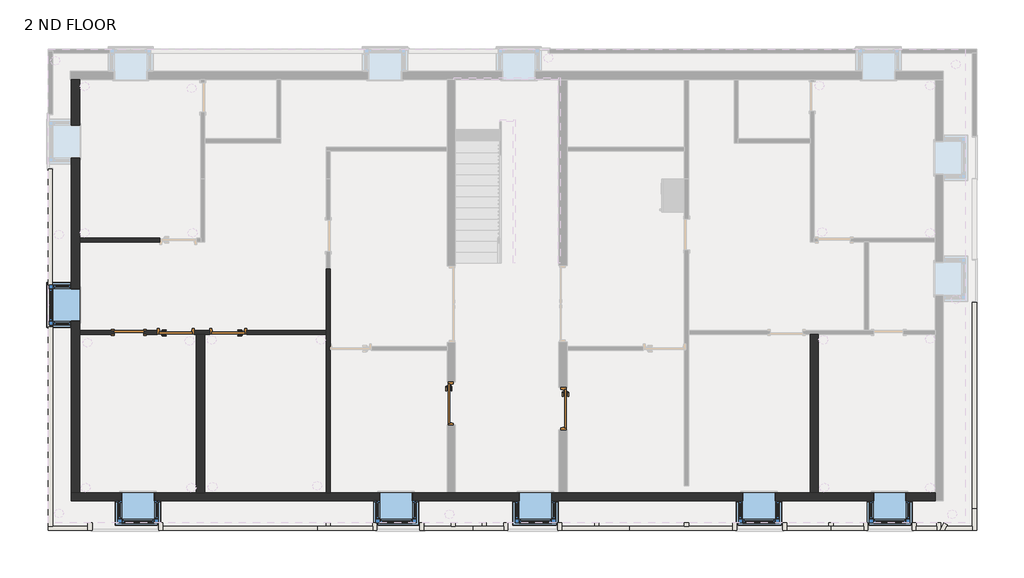
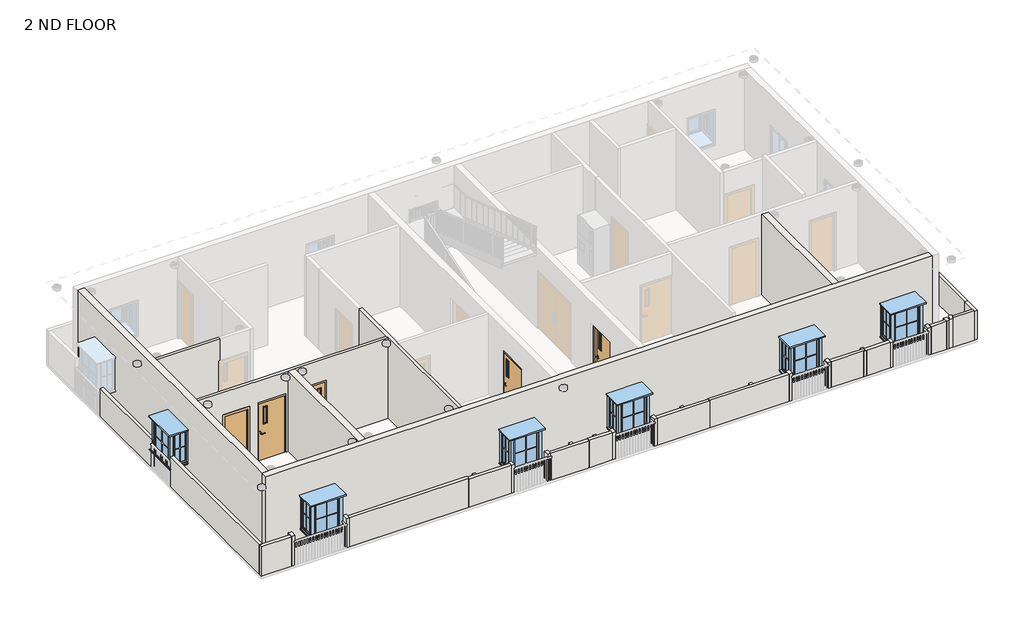
# One storey, part 1 of 7: 40 walls, 6 windows, 5 doors.
"""IFC4 building model written with IfcOpenShell, lengths in millimetres."""

from ifc_helpers import new_model, si_unit, frame, origin, place, context, project, spatial, polyline, outline, extrude, faceted_brep, transform, mapped, element, save
from components import door_586e558e, door_7d8f8091, door_passage_single_vision_lite_3_x7_440dd290, door_passage_single_vision_lite_3_x7_38248cdf, door_d141acb4, window_bay_casement_box_90_degree_angle_center_fixed_4_x3_2dea7aab

model = new_model("IFC4")

# Units and contexts
model_context = context("Model", 3, world=origin())
ifc_project = project(units=[si_unit("LENGTHUNIT", "METRE", prefix="MILLI")], contexts=[model_context])

# Site, building, storey
site = spatial("IfcSite", under=ifc_project)
building = spatial("IfcBuilding", under=site)
storey = spatial("IfcBuildingStorey", under=building, Name="2 ND FLOOR", Elevation=6400.8)

# Doors
placement = place(None, origin())
door_shape = door_586e558e(model_context)
element("IfcDoor", 1, ObjectType="Door-Passage-Single-Vision_Lite : 3'6\"X7' 2", at=placement, inside=storey, context=model_context, shape_type="MappedRepresentation", body=[
    mapped(door_shape, transform((1116.1432011, -1461.3932193, 6400.8), x_axis=(0.0, -1.0, 0.0), y_axis=(1.0, 0.0, 0.0), z_axis=(0.0, 0.0, 1.0))),
])
door_2_shape = door_7d8f8091(model_context)
element("IfcDoor", 2, ObjectType="Door-Passage-Single-Vision_Lite : 3'7\"X7' 3", at=placement, inside=storey, context=model_context, shape_type="MappedRepresentation", body=[
    mapped(door_2_shape, transform((-1956.7487998, -1318.7421379, 6400.8), x_axis=(0.0, -1.0, 0.0), y_axis=(1.0, 0.0, 0.0), z_axis=(0.0, 0.0, 1.0))),
])
door_passage_single_vision_lite_3_x7_shape = door_passage_single_vision_lite_3_x7_440dd290(model_context)
element("IfcDoor", 3, ObjectType="Door-Passage-Single-Vision_Lite : 3'X7'", at=placement, inside=storey, context=model_context, shape_type="MappedRepresentation", body=[
    mapped(door_passage_single_vision_lite_3_x7_shape, transform((-8122.5987992, 646.8067334, 6400.8), x_axis=(-1.0, 0.0, 0.0), y_axis=(0.0, -1.0, 0.0), z_axis=(0.0, 0.0, 1.0))),
])
door_passage_single_vision_lite_3_x7_2_shape = door_passage_single_vision_lite_3_x7_38248cdf(model_context)
element("IfcDoor", 4, ObjectType="Door-Passage-Single-Vision_Lite : 3'X7'", at=placement, inside=storey, context=model_context, shape_type="MappedRepresentation", body=[
    mapped(door_passage_single_vision_lite_3_x7_2_shape, transform((-9570.3987992, 646.8067334, 6400.8), x_axis=(1.0, 0.0, 0.0), y_axis=(0.0, 1.0, 0.0), z_axis=(0.0, 0.0, 1.0))),
])
door_3_shape = door_d141acb4(model_context)
element("IfcDoor", 5, ObjectType="Single-Flush : 2'8\"x 7'", at=placement, inside=storey, context=model_context, shape_type="MappedRepresentation", body=[
    mapped(door_3_shape, transform((-10865.7987992, 640.4567334, 6400.8), x_axis=(1.0, 0.0, 0.0), y_axis=(0.0, 1.0, 0.0), z_axis=(0.0, 0.0, 1.0))),
])

# Walls
element("IfcWall", 6, ObjectType="Generic - 4.5\"", at=placement, inside=storey, context=model_context, shape_type="SweptSolid", body=[
    extrude(outline(polyline([(9448.8, -9959.0462614), (9448.8, -12224.6987925), (6400.8, -12224.6987925), (6400.8, -10009.8462614), (8636.0, -10009.8462614), (8636.0, -9959.0462614), (9448.8, -9959.0462614)])), frame((0.0, 3136.0067332, 0.0), z_axis=(0.0, 1.0, 0.0), x_axis=(0.0, 0.0, 1.0)), (0.0, 0.0, 1.0), 114.3),
])
element("IfcWall", 7, ObjectType="Generic - 4.5\"", at=placement, inside=storey, context=model_context, shape_type="Brep", body=[
    faceted_brep([(-10459.3987992, 583.3067334, 8534.4), (-10459.3987992, 583.3067334, 6400.8), (-10078.3987992, 583.3067334, 6400.8), (-10078.3987992, 583.3067334, 8636.0), (-9062.3987992, 583.3067334, 8636.0), (-9062.3987992, 583.3067334, 6400.8), (-8998.8987992, 583.3067334, 6400.8), (-8770.2987992, 583.3067334, 6400.8), (-8630.5987992, 583.3067334, 6400.8), (-8630.5987992, 583.3067334, 8636.0), (-7614.5987992, 583.3067334, 8636.0), (-7614.5987992, 583.3067334, 6400.8), (-5417.4987995, 583.3067334, 6400.8), (-5417.4987995, 583.3067334, 9448.8), (-8770.2987992, 583.3067334, 9448.8), (-8998.8987992, 583.3067334, 9448.8), (-12224.6987925, 583.3067334, 9448.8), (-12224.6987925, 583.3067334, 6400.8), (-11272.1987992, 583.3067334, 6400.8), (-11272.1987992, 583.3067334, 8534.4), (-10078.3987992, 697.6067334, 6400.8), (-10459.3987992, 697.6067334, 6400.8), (-10459.3987992, 697.6067334, 8534.4), (-11272.1987992, 697.6067334, 8534.4), (-11272.1987992, 697.6067334, 6400.8), (-12224.6987925, 697.6067334, 6400.8), (-12224.6987925, 697.6067334, 9448.8), (-5417.4987995, 697.6067334, 9448.8), (-5417.4987995, 697.6067334, 6400.8), (-7614.5987992, 697.6067334, 6400.8), (-7614.5987992, 697.6067334, 8636.0), (-8630.5987992, 697.6067334, 8636.0), (-8630.5987992, 697.6067334, 6400.8), (-9062.3987992, 697.6067334, 6400.8), (-9062.3987992, 697.6067334, 8636.0), (-10078.3987992, 697.6067334, 8636.0)], [[[0, 1, 2, 3, 4, 5, 6, 7, 8, 9, 10, 11, 12, 13, 14, 15, 16, 17, 18, 19]], [[20, 21, 22, 23, 24, 25, 26, 27, 28, 29, 30, 31, 32, 33, 34, 35]], [[28, 12, 11, 29]], [[32, 8, 7, 6, 5, 33]], [[18, 17, 25, 24]], [[2, 1, 21, 20]], [[16, 15, 14, 13, 27, 26]], [[17, 16, 26, 25]], [[13, 12, 28, 27]], [[9, 8, 32, 31]], [[10, 9, 31, 30]], [[11, 10, 30, 29]], [[4, 34, 33, 5]], [[34, 4, 3, 35]], [[35, 3, 2, 20]], [[22, 21, 1, 0]], [[23, 22, 0, 19]], [[24, 23, 19, 18]]]),
])
element("IfcWall", 8, ObjectType="Generic - 4.5\"", at=placement, inside=storey, context=model_context, shape_type="Brep", body=[
    faceted_brep([(-5417.4987995, 2399.4067802, 6400.8), (-5417.4987995, 697.6067334, 6400.8), (-5417.4987995, 583.3067334, 6400.8), (-5417.4987995, -3785.4932193, 6400.8), (-5417.4987995, -3785.4932193, 9448.8), (-5417.4987995, 583.3067334, 9448.8), (-5417.4987995, 697.6067334, 9448.8), (-5417.4987995, 2399.4067802, 9448.8), (-5303.1987995, 2399.4067802, 9448.8), (-5303.1987995, 262.4078621, 9448.8), (-5303.1987995, 148.1078621, 9448.8), (-5303.1987995, -3785.4932193, 9448.8), (-5303.1987995, -3785.4932193, 6400.8), (-5303.1987995, 148.1078621, 6400.8), (-5303.1987995, 148.1078621, 8636.0), (-5303.1987995, 262.4078621, 8636.0), (-5303.1987995, 262.4078621, 6400.8), (-5303.1987995, 2399.4067802, 6400.8), (-5334.9487995, 262.4078621, 6400.8), (-5334.9487995, 148.1078621, 6400.8), (-5334.9487995, 262.4078621, 8636.0), (-5334.9487995, 148.1078621, 8636.0)], [[[0, 1, 2, 3, 4, 5, 6, 7]], [[8, 9, 10, 11, 12, 13, 14, 15, 16, 17]], [[3, 2, 1, 0, 17, 16, 18, 19, 13, 12]], [[7, 6, 5, 4, 11, 10, 9, 8]], [[0, 7, 8, 17]], [[20, 18, 16, 15]], [[19, 21, 14, 13]], [[21, 20, 15, 14]], [[18, 20, 21, 19]], [[4, 3, 12, 11]]]),
])
element("IfcWall", 9, ObjectType="Generic - 4.5\"", at=placement, inside=storey, context=model_context, shape_type="Brep", body=[
    faceted_brep([(-13088.8067989, -4826.8932661, 6400.8), (-11996.6067989, -4826.8932661, 6400.8), (-11996.6067989, -4826.8932661, 7513.7417562), (-13088.8067989, -4826.8932661, 7513.7417562), (-13088.8067989, -4712.5932661, 6400.8), (-13088.8067989, -4712.5932661, 7513.7417562), (-11996.6067989, -4712.5932661, 7513.7417562), (-11996.6067989, -4712.5932661, 6400.8), (-12974.5067989, -4712.5932661, 6400.8)], [[[0, 1, 2, 3]], [[4, 5, 6, 7, 8]], [[1, 0, 4, 8, 7]], [[3, 2, 6, 5]], [[2, 1, 7, 6]], [[0, 3, 5, 4]]]),
])
element("IfcWall", 10, ObjectType="Generic - 4.5\"", at=placement, inside=storey, context=model_context, shape_type="Brep", body=[
    faceted_brep([(-11996.6067989, -4623.6932193, 6400.8), (-11996.6067989, -4712.5932661, 6400.8), (-11996.6067989, -4826.8932661, 6400.8), (-11996.6067989, -4826.8932661, 7513.7417562), (-11996.6067989, -4826.8932661, 7534.7303619), (-11996.6067989, -4623.6932193, 7534.7303619), (-11882.3067989, -4623.6932193, 6400.8), (-11882.3067989, -4623.6932193, 7534.7303619), (-11882.3067989, -4826.8932661, 7534.7303619), (-11882.3067989, -4826.8932661, 6400.8)], [[[0, 1, 2, 3, 4, 5]], [[6, 7, 8, 9]], [[2, 1, 0, 6, 9]], [[5, 4, 8, 7]], [[0, 5, 7, 6]], [[4, 3, 2, 9, 8]]]),
])
element("IfcWall", 11, ObjectType="Generic - 4.5\"", at=placement, inside=storey, context=model_context, shape_type="Brep", body=[
    faceted_brep([(11660.3143245, -4826.8932661, 6400.8), (12426.0012043, -4826.8932661, 6400.8), (12426.0012043, -4826.8932661, 7492.6617784), (12426.0012043, -4826.8932661, 7503.9196614), (11660.3143245, -4826.8932661, 7503.9196614), (11660.3143245, -4826.8932661, 7490.3342527), (11716.0621594, -4712.5932661, 6400.8), (11716.0621594, -4712.5932661, 7503.9196614), (12426.0012043, -4712.5932661, 7503.9196614), (12426.0012043, -4712.5932661, 6400.8)], [[[0, 1, 2, 3, 4, 5]], [[6, 7, 8, 9]], [[1, 0, 6, 9]], [[4, 3, 8, 7]], [[3, 2, 1, 9, 8]], [[0, 5, 4, 7, 6]]]),
])
element("IfcWall", 12, ObjectType="Generic - 4.5\"", at=placement, inside=storey, context=model_context, shape_type="Brep", body=[
    faceted_brep([(11632.2512075, -4623.6932193, 6400.8), (11533.1439227, -4826.8932661, 6400.8), (11533.1439227, -4826.8932661, 7490.3342527), (11632.2512075, -4623.6932193, 7490.3342527), (11734.983367, -4673.7990414, 6400.8), (11734.983367, -4673.7990414, 7490.3342527), (11660.3143245, -4826.8932661, 7490.3342527), (11660.3143245, -4826.8932661, 6400.8), (11716.0621594, -4712.5932661, 6400.8)], [[[0, 1, 2, 3]], [[4, 5, 6, 7, 8]], [[1, 0, 4, 8, 7]], [[3, 2, 6, 5]], [[0, 3, 5, 4]], [[2, 1, 7, 6]]]),
])
element("IfcWall", 13, ObjectType="Generic - 4.5\"", at=placement, inside=storey, context=model_context, shape_type="Brep", body=[
    faceted_brep([(12426.0012043, -4236.3432661, 6400.8), (12426.0012043, -4712.5932661, 6400.8), (12426.0012043, -4826.8932661, 6400.8), (12426.0012043, -4826.8932661, 7492.6617784), (12426.0012043, -4236.3432661, 7492.6617784), (12426.0012043, -4236.3432661, 7487.4712164), (12540.3012043, -4236.3432661, 6400.8), (12540.3012043, -4236.3432661, 7487.4712164), (12540.3012043, -4236.3432661, 7492.6617784), (12540.3012043, -4826.8932661, 7492.6617784), (12540.3012043, -4826.8932661, 6400.8)], [[[0, 1, 2, 3, 4, 5]], [[6, 7, 8, 9, 10]], [[2, 1, 0, 6, 10]], [[4, 3, 9, 8]], [[0, 5, 4, 8, 7, 6]], [[3, 2, 10, 9]]]),
])
element("IfcWall", 14, ObjectType="Generic - 4.5\"", at=placement, inside=storey, context=model_context, shape_type="SweptSolid", body=[
    extrude(outline(polyline([(-5417.4987995, -4712.5932661), (-5417.4987995, -4623.6932193), (-5303.1987995, -4623.6932193), (-5303.1987995, -4712.5932661), (-5417.4987995, -4712.5932661)])), frame((0.0, 0.0, 6400.8), z_axis=(0.0, 0.0, 1.0), x_axis=(1.0, 0.0, 0.0)), (0.0, 0.0, 1.0), 1063.0786215),
])
element("IfcWall", 15, ObjectType="Generic - 4.5\"", at=placement, inside=storey, context=model_context, shape_type="Brep", body=[
    faceted_brep([(-5663.8033402, -4826.8932661, 6400.8), (-4134.7987995, -4826.8932661, 6400.8), (-4134.7987995, -4826.8932661, 7459.9218247), (-4134.7987995, -4826.8932661, 7468.0575049), (-5663.8033402, -4826.8932661, 7468.0575049), (-5663.8033402, -4712.5932661, 6400.8), (-5663.8033402, -4712.5932661, 7468.0575049), (-4134.7987995, -4712.5932661, 7468.0575049), (-4134.7987995, -4712.5932661, 6400.8), (-5303.1987995, -4712.5932661, 6400.8), (-5417.4987995, -4712.5932661, 6400.8)], [[[0, 1, 2, 3, 4]], [[5, 6, 7, 8, 9, 10]], [[1, 0, 5, 10, 9, 8]], [[4, 3, 7, 6]], [[0, 4, 6, 5]], [[3, 2, 1, 8, 7]]]),
])
element("IfcWall", 16, ObjectType="Generic - 4.5\"", at=placement, inside=storey, context=model_context, shape_type="Brep", body=[
    faceted_brep([(-2725.0987995, -4826.8932661, 6400.8), (-1354.4417672, -4826.8932661, 6400.8), (-1354.4417672, -4826.8932661, 7416.8), (-2725.0987995, -4826.8932661, 7416.8), (-2725.0987995, -4712.5932661, 6400.8), (-2725.0987995, -4712.5932661, 7416.8), (-1354.4417672, -4712.5932661, 7416.8), (-1354.4417672, -4712.5932661, 6400.8), (-1848.7987998, -4712.5932661, 6400.8), (-1963.0987998, -4712.5932661, 6400.8)], [[[0, 1, 2, 3]], [[4, 5, 6, 7, 8, 9]], [[1, 0, 4, 9, 8, 7]], [[2, 1, 7, 6]], [[3, 2, 6, 5]], [[0, 3, 5, 4]]]),
])
element("IfcWall", 17, ObjectType="Generic - 4.5\"", at=placement, inside=storey, context=model_context, shape_type="SweptSolid", body=[
    extrude(outline(polyline([(-1963.0987998, -4712.5932661), (-1963.0987998, -4623.6932193), (-1848.7987998, -4623.6932193), (-1848.7987998, -4712.5932661), (-1963.0987998, -4712.5932661)])), frame((0.0, 0.0, 6400.8), z_axis=(0.0, 0.0, 1.0), x_axis=(1.0, 0.0, 0.0)), (0.0, 0.0, 1.0), 1029.3234006),
])
element("IfcWall", 18, ObjectType="Generic - 4.5\"", at=placement, inside=storey, context=model_context, shape_type="SweptSolid", body=[
    extrude(outline(polyline([(-1112.1987998, -4712.5932661), (-1112.1987998, -4623.6932193), (-997.8987998, -4623.6932193), (-997.8987998, -4712.5932661), (-1112.1987998, -4712.5932661)])), frame((0.0, 0.0, 6400.8), z_axis=(0.0, 0.0, 1.0), x_axis=(1.0, 0.0, 0.0)), (0.0, 0.0, 1.0), 1016.0),
])
element("IfcWall", 19, ObjectType="Generic - 4.5\"", at=placement, inside=storey, context=model_context, shape_type="SweptSolid", body=[
    extrude(outline(polyline([(1999.3012002, -4712.5932661), (1999.3012002, -4623.6932193), (2113.6012002, -4623.6932193), (2113.6012002, -4712.5932661), (1999.3012002, -4712.5932661)])), frame((0.0, 0.0, 6400.8), z_axis=(0.0, 0.0, 1.0), x_axis=(1.0, 0.0, 0.0)), (0.0, 0.0, 1.0), 1013.2250283),
])
element("IfcWall", 20, ObjectType="Generic - 4.5\"", at=placement, inside=storey, context=model_context, shape_type="SweptSolid", body=[
    extrude(outline(polyline([(4475.8012082, -4712.5932661), (4475.8012082, -4623.6932193), (4590.1012082, -4623.6932193), (4590.1012082, -4712.5932661), (4475.8012082, -4712.5932661)])), frame((0.0, 0.0, 6400.8), z_axis=(0.0, 0.0, 1.0), x_axis=(1.0, 0.0, 0.0)), (0.0, 0.0, 1.0), 1027.4591445),
])
element("IfcWall", 21, ObjectType="Generic - 4.5\"", at=placement, inside=storey, context=model_context, shape_type="Brep", body=[
    faceted_brep([(2962.6087812, -4826.8932661, 6400.8), (5802.9512082, -4826.8932661, 6400.8), (5802.9512082, -4826.8932661, 7428.2591445), (2962.6087812, -4826.8932661, 7428.2591445), (2962.6087812, -4826.8932661, 7414.0250283), (2962.6087812, -4712.5932661, 6400.8), (2962.6087812, -4712.5932661, 7414.0250283), (2962.6087812, -4712.5932661, 7428.2591445), (4475.8012082, -4712.5932661, 7428.2591445), (4590.1012082, -4712.5932661, 7428.2591445), (5802.9512082, -4712.5932661, 7428.2591445), (5802.9512082, -4712.5932661, 6400.8), (4590.1012082, -4712.5932661, 6400.8), (4475.8012082, -4712.5932661, 6400.8)], [[[0, 1, 2, 3, 4]], [[5, 6, 7, 8, 9, 10, 11, 12, 13]], [[1, 0, 5, 13, 12, 11]], [[3, 2, 10, 9, 8, 7]], [[0, 4, 3, 7, 6, 5]], [[2, 1, 11, 10]]]),
])
element("IfcWall", 22, ObjectType="Generic - 4.5\"", at=placement, inside=storey, context=model_context, shape_type="Brep", body=[
    faceted_brep([(5802.9512082, -4623.6932193, 6400.8), (5802.9512082, -4712.5932661, 6400.8), (5802.9512082, -4826.8932661, 6400.8), (5802.9512082, -4826.8932661, 7428.2591445), (5802.9512082, -4826.8932661, 7433.1822201), (5802.9512082, -4623.6932193, 7433.1822201), (5917.2512082, -4623.6932193, 6400.8), (5917.2512082, -4623.6932193, 7433.1822201), (5917.2512082, -4826.8932661, 7433.1822201), (5917.2512082, -4826.8932661, 6400.8)], [[[0, 1, 2, 3, 4, 5]], [[6, 7, 8, 9]], [[2, 1, 0, 6, 9]], [[5, 4, 8, 7]], [[0, 5, 7, 6]], [[4, 3, 2, 9, 8]]]),
])
element("IfcWall", 23, ObjectType="Generic - 4.5\"", at=placement, inside=storey, context=model_context, shape_type="Brep", body=[
    faceted_brep([(7190.3011643, -4623.6932193, 6400.8), (7190.3011643, -4826.8932661, 6400.8), (7190.3011643, -4826.8932661, 7373.6158009), (7190.3011643, -4623.6932193, 7373.6158009), (7304.6011643, -4623.6932193, 6400.8), (7304.6011643, -4623.6932193, 7373.6158009), (7304.6011643, -4712.5932661, 7373.6158009), (7304.6011643, -4826.8932661, 7373.6158009), (7304.6011643, -4826.8932661, 6400.8), (7304.6011643, -4712.5932661, 6400.8)], [[[0, 1, 2, 3]], [[4, 5, 6, 7, 8, 9]], [[1, 0, 4, 9, 8]], [[3, 2, 7, 6, 5]], [[0, 3, 5, 4]], [[2, 1, 8, 7]]]),
])
element("IfcWall", 24, ObjectType="Generic - 4.5\"", at=placement, inside=storey, context=model_context, shape_type="Brep", body=[
    faceted_brep([(7304.6011643, -4826.8932661, 6400.8), (8463.6012082, -4826.8932661, 6400.8), (8463.6012082, -4826.8932661, 7357.2159658), (8520.7512082, -4826.8932661, 7357.2159658), (8520.7512082, -4826.8932661, 7370.480309), (8520.7512082, -4826.8932661, 7373.7581334), (7304.6011643, -4826.8932661, 7373.7581334), (7304.6011643, -4712.5932661, 6400.8), (7304.6011643, -4712.5932661, 7373.7581334), (8520.7512082, -4712.5932661, 7373.7581334), (8520.7512082, -4712.5932661, 7370.480309), (8520.7512082, -4712.5932661, 7357.2159658), (8463.6012082, -4712.5932661, 7357.2159658), (8463.6012082, -4712.5932661, 6400.8)], [[[0, 1, 2, 3, 4, 5, 6]], [[7, 8, 9, 10, 11, 12, 13]], [[1, 0, 7, 13]], [[6, 5, 9, 8]], [[0, 6, 8, 7]], [[5, 4, 3, 11, 10, 9]], [[11, 3, 2, 12]], [[2, 1, 13, 12]]]),
])
element("IfcWall", 25, ObjectType="Generic - 4.5\"", at=placement, inside=storey, context=model_context, shape_type="Brep", body=[
    faceted_brep([(8463.6012082, -4623.6932193, 6400.8), (8463.6012082, -4712.5932661, 6400.8), (8463.6012082, -4826.8932661, 6400.8), (8463.6012082, -4826.8932661, 7357.2159658), (8463.6012082, -4712.5932661, 7357.2159658), (8463.6012082, -4623.6932193, 7357.2159658), (8577.9012082, -4623.6932193, 6400.8), (8577.9012082, -4623.6932193, 7357.2159658), (8577.9012082, -4712.5932661, 7357.2159658), (8577.9012082, -4826.8932661, 7357.2159658), (8577.9012082, -4826.8932661, 6400.8), (8577.9012082, -4712.5932661, 6400.8), (8520.7512082, -4826.8932661, 7357.2159658)], [[[0, 1, 2, 3, 4, 5]], [[6, 7, 8, 9, 10, 11]], [[2, 1, 0, 6, 11, 10]], [[5, 4, 3, 12, 9, 8, 7]], [[0, 5, 7, 6]], [[3, 2, 10, 9, 12]]]),
])
element("IfcWall", 26, ObjectType="Generic - 4.5\"", at=placement, inside=storey, context=model_context, shape_type="Brep", body=[
    faceted_brep([(8577.9012082, -4826.8932661, 6400.8), (9422.4512082, -4826.8932661, 6400.8), (9422.4512082, -4826.8932661, 7353.0060641), (9422.4512082, -4826.8932661, 7370.480309), (8520.7512082, -4826.8932661, 7370.480309), (8520.7512082, -4826.8932661, 7357.2159658), (8577.9012082, -4826.8932661, 7357.2159658), (8577.9012082, -4712.5932661, 6400.8), (8577.9012082, -4712.5932661, 7357.2159658), (8520.7512082, -4712.5932661, 7357.2159658), (8520.7512082, -4712.5932661, 7370.480309), (9422.4512082, -4712.5932661, 7370.480309), (9422.4512082, -4712.5932661, 6400.8)], [[[0, 1, 2, 3, 4, 5, 6]], [[7, 8, 9, 10, 11, 12]], [[1, 0, 7, 12]], [[4, 3, 11, 10]], [[3, 2, 1, 12, 11]], [[5, 4, 10, 9]], [[5, 9, 8, 6]], [[0, 6, 8, 7]]]),
])
element("IfcWall", 27, ObjectType="Generic - 4.5\"", at=placement, inside=storey, context=model_context, shape_type="Brep", body=[
    faceted_brep([(9422.4512082, -4623.6932193, 6400.8), (9422.4512082, -4712.5932661, 6400.8), (9422.4512082, -4826.8932661, 6400.8), (9422.4512082, -4826.8932661, 7353.0060641), (9422.4512082, -4623.6932193, 7353.0060641), (9536.7512082, -4623.6932193, 6400.8), (9536.7512082, -4623.6932193, 7353.0060641), (9536.7512082, -4826.8932661, 7353.0060641), (9536.7512082, -4826.8932661, 6400.8)], [[[0, 1, 2, 3, 4]], [[5, 6, 7, 8]], [[2, 1, 0, 5, 8]], [[4, 3, 7, 6]], [[0, 4, 6, 5]], [[3, 2, 8, 7]]]),
])
element("IfcWall", 28, ObjectType="Generic - 4.5\"", at=placement, inside=storey, context=model_context, shape_type="Brep", body=[
    faceted_brep([(10764.1617205, -4623.6932193, 6400.8), (10764.1617205, -4826.8932661, 6400.8), (10764.1617205, -4826.8932661, 7427.1072304), (10764.1617205, -4623.6932193, 7427.1072304), (10878.4617205, -4623.6932193, 6400.8), (10878.4617205, -4623.6932193, 7427.1072304), (10878.4617205, -4826.8932661, 7427.1072304), (10878.4617205, -4826.8932661, 6400.8), (10878.4617205, -4712.5932661, 6400.8)], [[[0, 1, 2, 3]], [[4, 5, 6, 7, 8]], [[1, 0, 4, 8, 7]], [[3, 2, 6, 5]], [[0, 3, 5, 4]], [[2, 1, 7, 6]]]),
])
element("IfcWall", 29, ObjectType="Generic - 4.5\"", at=placement, inside=storey, context=model_context, shape_type="Brep", body=[
    faceted_brep([(10878.4617205, -4826.8932661, 6400.8), (11437.2617205, -4826.8932661, 6400.8), (11437.2617205, -4826.8932661, 7449.4912221), (10878.4617205, -4826.8932661, 7449.4912221), (10878.4617205, -4826.8932661, 7427.1072304), (10878.4617205, -4712.5932661, 6400.8), (10878.4617205, -4712.5932661, 7449.4912221), (11437.2617205, -4712.5932661, 7449.4912221), (11437.2617205, -4712.5932661, 6400.8)], [[[0, 1, 2, 3, 4]], [[5, 6, 7, 8]], [[1, 0, 5, 8]], [[3, 2, 7, 6]], [[0, 4, 3, 6, 5]], [[2, 1, 8, 7]]]),
])
element("IfcWall", 30, ObjectType="Generic - 4.5\"", at=placement, inside=storey, context=model_context, shape_type="Brep", body=[
    faceted_brep([(11437.2617205, -4623.6932193, 6400.8), (11437.2617205, -4712.5932661, 6400.8), (11437.2617205, -4826.8932661, 6400.8), (11437.2617205, -4826.8932661, 7449.4912221), (11437.2617205, -4712.5932661, 7449.4912221), (11437.2617205, -4623.6932193, 7449.4912221), (11551.5617205, -4623.6932193, 6400.8), (11551.5617205, -4623.6932193, 7449.4912221), (11551.5617205, -4826.8932661, 7449.4912221), (11551.5617205, -4826.8932661, 6400.8)], [[[0, 1, 2, 3, 4, 5]], [[6, 7, 8, 9]], [[2, 1, 0, 6, 9]], [[5, 4, 3, 8, 7]], [[0, 5, 7, 6]], [[3, 2, 9, 8]]]),
])
element("IfcWall", 31, ObjectType="Generic - 4.5\"", at=placement, inside=storey, context=model_context, shape_type="Brep", body=[
    faceted_brep([(-4134.7987995, -4623.6932193, 6400.8), (-4134.7987995, -4712.5932661, 6400.8), (-4134.7987995, -4826.8932661, 6400.8), (-4134.7987995, -4826.8932661, 7459.9218247), (-4134.7987995, -4623.6932193, 7459.9218247), (-4020.4987995, -4623.6932193, 6400.8), (-4020.4987995, -4623.6932193, 7459.9218247), (-4020.4987995, -4826.8932661, 7459.9218247), (-4020.4987995, -4826.8932661, 6400.8)], [[[0, 1, 2, 3, 4]], [[5, 6, 7, 8]], [[2, 1, 0, 5, 8]], [[4, 3, 7, 6]], [[0, 4, 6, 5]], [[3, 2, 8, 7]]]),
])
element("IfcWall", 32, ObjectType="Generic - 4.5\"", at=placement, inside=storey, context=model_context, shape_type="Brep", body=[
    faceted_brep([(-2839.3987995, -4623.6932193, 6400.8), (-2839.3987995, -4826.8932661, 6400.8), (-2839.3987995, -4826.8932661, 7417.5549618), (-2839.3987995, -4623.6932193, 7417.5549618), (-2725.0987995, -4623.6932193, 6400.8), (-2725.0987995, -4623.6932193, 7417.5549618), (-2725.0987995, -4826.8932661, 7417.5549618), (-2725.0987995, -4826.8932661, 7416.8), (-2725.0987995, -4826.8932661, 6400.8), (-2725.0987995, -4712.5932661, 6400.8)], [[[0, 1, 2, 3]], [[4, 5, 6, 7, 8, 9]], [[1, 0, 4, 9, 8]], [[3, 2, 6, 5]], [[0, 3, 5, 4]], [[2, 1, 8, 7, 6]]]),
])
element("IfcWall", 33, ObjectType="Generic - 4.5\"", at=placement, inside=storey, context=model_context, shape_type="Brep", body=[
    faceted_brep([(-1354.4417672, -4826.8932661, 6400.8), (-520.5065315, -4826.8932661, 6400.8), (-520.5065315, -4826.8932661, 7424.6796817), (-520.5065315, -4826.8932661, 7431.940074), (-1354.4417672, -4826.8932661, 7431.940074), (-1354.4417672, -4826.8932661, 7416.8), (-1354.4417672, -4712.5932661, 6400.8), (-1354.4417672, -4712.5932661, 7416.8), (-1354.4417672, -4712.5932661, 7431.940074), (-520.5065315, -4712.5932661, 7431.940074), (-520.5065315, -4712.5932661, 6400.8), (-997.8987998, -4712.5932661, 6400.8), (-1112.1987998, -4712.5932661, 6400.8)], [[[0, 1, 2, 3, 4, 5]], [[6, 7, 8, 9, 10, 11, 12]], [[1, 0, 6, 12, 11, 10]], [[4, 3, 9, 8]], [[0, 5, 4, 8, 7, 6]], [[3, 2, 1, 10, 9]]]),
])
element("IfcWall", 34, ObjectType="Generic - 4.5\"", at=placement, inside=storey, context=model_context, shape_type="Brep", body=[
    faceted_brep([(-520.5065315, -4623.6932193, 6400.8), (-520.5065315, -4712.5932661, 6400.8), (-520.5065315, -4826.8932661, 6400.8), (-520.5065315, -4826.8932661, 7424.6796817), (-520.5065315, -4623.6932193, 7424.6796817), (-406.2065315, -4623.6932193, 6400.8), (-406.2065315, -4623.6932193, 7424.6796817), (-406.2065315, -4826.8932661, 7424.6796817), (-406.2065315, -4826.8932661, 6400.8)], [[[0, 1, 2, 3, 4]], [[5, 6, 7, 8]], [[2, 1, 0, 5, 8]], [[4, 3, 7, 6]], [[0, 4, 6, 5]], [[3, 2, 8, 7]]]),
])
element("IfcWall", 35, ObjectType="Generic - 4.5\"", at=placement, inside=storey, context=model_context, shape_type="Brep", body=[
    faceted_brep([(970.0932011, -4623.6932193, 6400.8), (970.0932011, -4826.8932661, 6400.8), (970.0932011, -4826.8932661, 7414.0250283), (970.0932011, -4623.6932193, 7414.0250283), (1084.3932011, -4623.6932193, 6400.8), (1084.3932011, -4623.6932193, 7414.0250283), (1084.3932011, -4712.5932661, 7414.0250283), (1084.3932011, -4826.8932661, 7414.0250283), (1084.3932011, -4826.8932661, 6400.8), (1084.3932011, -4712.5932661, 6400.8)], [[[0, 1, 2, 3]], [[4, 5, 6, 7, 8, 9]], [[1, 0, 4, 9, 8]], [[3, 2, 7, 6, 5]], [[0, 3, 5, 4]], [[2, 1, 8, 7]]]),
])
element("IfcWall", 36, ObjectType="Generic - 4.5\"", at=placement, inside=storey, context=model_context, shape_type="Brep", body=[
    faceted_brep([(1084.3932011, -4826.8932661, 6400.8), (2962.6087812, -4826.8932661, 6400.8), (2962.6087812, -4826.8932661, 7414.0250283), (1084.3932011, -4826.8932661, 7414.0250283), (1084.3932011, -4712.5932661, 6400.8), (1084.3932011, -4712.5932661, 7414.0250283), (1999.3012002, -4712.5932661, 7414.0250283), (2113.6012002, -4712.5932661, 7414.0250283), (2962.6087812, -4712.5932661, 7414.0250283), (2962.6087812, -4712.5932661, 6400.8), (2113.6012002, -4712.5932661, 6400.8), (1999.3012002, -4712.5932661, 6400.8)], [[[0, 1, 2, 3]], [[4, 5, 6, 7, 8, 9, 10, 11]], [[1, 0, 4, 11, 10, 9]], [[2, 1, 9, 8]], [[3, 2, 8, 7, 6, 5]], [[0, 3, 5, 4]]]),
])
element("IfcWall", 37, ObjectType="Generic - 4.5\"", at=placement, inside=storey, context=model_context, shape_type="Brep", body=[
    faceted_brep([(-10045.9470335, -4623.6932193, 6400.8), (-10045.9470335, -4826.8932661, 6400.8), (-10045.9470335, -4826.8932661, 7508.504535), (-10045.9470335, -4623.6932193, 7508.504535), (-9931.6470335, -4623.6932193, 6400.8), (-9931.6470335, -4623.6932193, 7508.504535), (-9931.6470335, -4712.5932661, 7508.504535), (-9931.6470335, -4826.8932661, 7508.504535), (-9931.6470335, -4826.8932661, 6400.8), (-9931.6470335, -4712.5932661, 6400.8)], [[[0, 1, 2, 3]], [[4, 5, 6, 7, 8, 9]], [[1, 0, 4, 9, 8]], [[3, 2, 7, 6, 5]], [[0, 3, 5, 4]], [[2, 1, 8, 7]]]),
])
element("IfcWall", 38, ObjectType="Generic - 4.5\"", at=placement, inside=storey, context=model_context, shape_type="Brep", body=[
    faceted_brep([(-9931.6470335, -4826.8932661, 6400.8), (-5663.8033402, -4826.8932661, 6400.8), (-5663.8033402, -4826.8932661, 7468.0575049), (-5663.8033402, -4826.8932661, 7508.504535), (-9931.6470335, -4826.8932661, 7508.504535), (-9931.6470335, -4712.5932661, 6400.8), (-9931.6470335, -4712.5932661, 7508.504535), (-5663.8033402, -4712.5932661, 7508.504535), (-5663.8033402, -4712.5932661, 7468.0575049), (-5663.8033402, -4712.5932661, 6400.8)], [[[0, 1, 2, 3, 4]], [[5, 6, 7, 8, 9]], [[1, 0, 5, 9]], [[3, 2, 1, 9, 8, 7]], [[4, 3, 7, 6]], [[0, 4, 6, 5]]]),
])
element("IfcWall", 39, ObjectType="Generic - 4.5\"", at=placement, inside=storey, context=model_context, shape_type="Brep", body=[
    faceted_brep([(-13088.8067989, 792.8567339, 6400.8), (-13088.8067989, -4712.5932661, 6400.8), (-13088.8067989, -4712.5932661, 7513.7417562), (-13088.8067989, -4712.5932661, 7514.967936), (-13088.8067989, 792.8567339, 7514.967936), (-12974.5067989, 792.8567339, 6400.8), (-12974.5067989, 792.8567339, 7514.967936), (-12974.5067989, -4712.5932661, 7514.967936), (-12974.5067989, -4712.5932661, 6400.8)], [[[0, 1, 2, 3, 4]], [[5, 6, 7, 8]], [[1, 0, 5, 8]], [[4, 3, 7, 6]], [[0, 4, 6, 5]], [[3, 2, 1, 8, 7]]]),
])
element("IfcWall", 40, ObjectType="Generic - 4.5\"", at=placement, inside=storey, context=model_context, shape_type="SweptSolid", body=[
    extrude(outline(polyline([(-12976.0338648, 5154.3604213), (-12976.0338648, 1953.9604213), (-13090.3338648, 1953.9604213), (-13090.3338648, 5154.3604213), (-12976.0338648, 5154.3604213)])), frame((0.0, 0.0, 6400.8), z_axis=(0.0, 0.0, 1.0), x_axis=(1.0, 0.0, 0.0)), (0.0, 0.0, 1.0), 1047.4413329),
])
element("IfcWall", 41, ObjectType="Generic - 4.5\"", at=placement, inside=storey, context=model_context, shape_type="SweptSolid", body=[
    extrude(outline(polyline([(12426.0012043, -4236.3432661), (12426.0012043, 1478.6567334), (12540.3012043, 1478.6567334), (12540.3012043, -4236.3432661), (12426.0012043, -4236.3432661)])), frame((0.0, 0.0, 6400.8), z_axis=(0.0, 0.0, 1.0), x_axis=(1.0, 0.0, 0.0)), (0.0, 0.0, 1.0), 1086.6712164),
])
element("IfcWall", 42, ObjectType="Generic - 9\"", at=placement, inside=storey, context=model_context, shape_type="Brep", body=[
    faceted_brep([(11397.3012075, -3785.4932193, 6400.8), (8171.5012079, -3785.4932193, 6400.8), (7942.9012079, -3785.4932193, 6400.8), (1236.7932011, -3785.4932193, 6400.8), (1008.1932011, -3785.4932193, 6400.8), (-1848.7987998, -3785.4932193, 6400.8), (-2077.3987998, -3785.4932193, 6400.8), (-5303.1987995, -3785.4932193, 6400.8), (-5417.4987995, -3785.4932193, 6400.8), (-8770.2987992, -3785.4932193, 6400.8), (-8998.8987992, -3785.4932193, 6400.8), (-12224.6987925, -3785.4932193, 6400.8), (-12453.2987925, -3785.4932193, 6400.8), (-12453.2987925, -3785.4932193, 9448.8), (-12224.6987925, -3785.4932193, 9448.8), (-8998.8987992, -3785.4932193, 9448.8), (-8770.2987992, -3785.4932193, 9448.8), (-5417.4987995, -3785.4932193, 9448.8), (-5303.1987995, -3785.4932193, 9448.8), (-2077.3987998, -3785.4932193, 9448.8), (-1848.7987998, -3785.4932193, 9448.8), (1008.1932011, -3785.4932193, 9448.8), (1236.7932011, -3785.4932193, 9448.8), (7942.9012079, -3785.4932193, 9448.8), (8171.5012079, -3785.4932193, 9448.8), (11397.3012075, -3785.4932193, 9448.8), (-11068.9987958, -3785.4932193, 8280.4), (-11068.9987958, -3785.4932193, 7010.4), (-10154.5987958, -3785.4932193, 7010.4), (-10154.5987958, -3785.4932193, 8280.4), (-3944.2987998, -3785.4932193, 8280.4), (-3944.2987998, -3785.4932193, 7010.4), (-3029.8987998, -3785.4932193, 7010.4), (-3029.8987998, -3785.4932193, 8280.4), (-96.7067989, -3785.4932193, 8280.4), (-96.7067989, -3785.4932193, 7010.4), (817.6932011, -3785.4932193, 7010.4), (817.6932011, -3785.4932193, 8280.4), (6076.0012079, -3785.4932193, 8280.4), (6076.0012079, -3785.4932193, 7010.4), (6990.4012079, -3785.4932193, 7010.4), (6990.4012079, -3785.4932193, 8280.4), (9682.8012075, -3785.4932193, 8280.4), (9682.8012075, -3785.4932193, 7010.4), (10597.2012075, -3785.4932193, 7010.4), (10597.2012075, -3785.4932193, 8280.4), (11397.3012075, -4014.0932193, 6400.8), (11397.3012075, -4014.0932193, 9448.8), (-12453.2987925, -4014.0932193, 9448.8), (-12453.2987925, -4014.0932193, 6400.8), (-11068.9987958, -4014.0932193, 8280.4), (-10154.5987958, -4014.0932193, 8280.4), (-10154.5987958, -4014.0932193, 7010.4), (-11068.9987958, -4014.0932193, 7010.4), (-3944.2987998, -4014.0932193, 8280.4), (-3029.8987998, -4014.0932193, 8280.4), (-3029.8987998, -4014.0932193, 7010.4), (-3944.2987998, -4014.0932193, 7010.4), (-96.7067989, -4014.0932193, 8280.4), (817.6932011, -4014.0932193, 8280.4), (817.6932011, -4014.0932193, 7010.4), (-96.7067989, -4014.0932193, 7010.4), (6076.0012079, -4014.0932193, 8280.4), (6990.4012079, -4014.0932193, 8280.4), (6990.4012079, -4014.0932193, 7010.4), (6076.0012079, -4014.0932193, 7010.4), (9682.8012075, -4014.0932193, 8280.4), (10597.2012075, -4014.0932193, 8280.4), (10597.2012075, -4014.0932193, 7010.4), (9682.8012075, -4014.0932193, 7010.4)], [[[0, 1, 2, 3, 4, 5, 6, 7, 8, 9, 10, 11, 12, 13, 14, 15, 16, 17, 18, 19, 20, 21, 22, 23, 24, 25], [26, 27, 28, 29], [30, 31, 32, 33], [34, 35, 36, 37], [38, 39, 40, 41], [42, 43, 44, 45]], [[46, 47, 48, 49], [50, 51, 52, 53], [54, 55, 56, 57], [58, 59, 60, 61], [62, 63, 64, 65], [66, 67, 68, 69]], [[12, 11, 10, 9, 8, 7, 6, 5, 4, 3, 2, 1, 0, 46, 49]], [[25, 24, 23, 22, 21, 20, 19, 18, 17, 16, 15, 14, 13, 48, 47]], [[0, 25, 47, 46]], [[13, 12, 49, 48]], [[27, 26, 50, 53]], [[28, 27, 53, 52]], [[29, 28, 52, 51]], [[26, 29, 51, 50]], [[31, 30, 54, 57]], [[32, 31, 57, 56]], [[33, 32, 56, 55]], [[30, 33, 55, 54]], [[35, 34, 58, 61]], [[36, 35, 61, 60]], [[37, 36, 60, 59]], [[34, 37, 59, 58]], [[39, 38, 62, 65]], [[40, 39, 65, 64]], [[41, 40, 64, 63]], [[38, 41, 63, 62]], [[43, 42, 66, 69]], [[44, 43, 69, 68]], [[45, 44, 68, 67]], [[42, 45, 67, 66]]]),
])
element("IfcWall", 43, ObjectType="Generic - 9\"", at=placement, inside=storey, context=model_context, shape_type="Brep", body=[
    faceted_brep([(-12224.6987925, -3785.4932193, 6400.8), (-12224.6987925, 583.3067334, 6400.8), (-12224.6987925, 697.6067334, 6400.8), (-12224.6987925, 3136.0067332, 6400.8), (-12224.6987925, 3250.3067332, 6400.8), (-12224.6987925, 7631.8067329, 6400.8), (-12224.6987925, 7631.8067329, 9448.8), (-12224.6987925, 3250.3067332, 9448.8), (-12224.6987925, 3136.0067332, 9448.8), (-12224.6987925, 697.6067334, 9448.8), (-12224.6987925, 583.3067334, 9448.8), (-12224.6987925, -3785.4932193, 9448.8), (-12224.6987925, 1859.6567334, 8280.4), (-12224.6987925, 1859.6567334, 7010.4), (-12224.6987925, 945.2567334, 7010.4), (-12224.6987925, 945.2567334, 8280.4), (-12224.6987925, 6374.5067329, 8280.4), (-12224.6987925, 6374.5067329, 7010.4), (-12224.6987925, 5460.1067329, 7010.4), (-12224.6987925, 5460.1067329, 8280.4), (-12453.2987925, -3785.4932193, 6400.8), (-12453.2987925, -3785.4932193, 9448.8), (-12453.2987925, 7631.8067329, 9448.8), (-12453.2987925, 7631.8067329, 6400.8), (-12453.2987925, 1859.6567334, 8280.4), (-12453.2987925, 945.2567334, 8280.4), (-12453.2987925, 945.2567334, 7010.4), (-12453.2987925, 1859.6567334, 7010.4), (-12453.2987925, 6374.5067329, 8280.4), (-12453.2987925, 5460.1067329, 8280.4), (-12453.2987925, 5460.1067329, 7010.4), (-12453.2987925, 6374.5067329, 7010.4)], [[[0, 1, 2, 3, 4, 5, 6, 7, 8, 9, 10, 11], [12, 13, 14, 15], [16, 17, 18, 19]], [[20, 21, 22, 23], [24, 25, 26, 27], [28, 29, 30, 31]], [[5, 4, 3, 2, 1, 0, 20, 23]], [[11, 10, 9, 8, 7, 6, 22, 21]], [[0, 11, 21, 20]], [[6, 5, 23, 22]], [[13, 12, 24, 27]], [[14, 13, 27, 26]], [[15, 14, 26, 25]], [[12, 15, 25, 24]], [[17, 16, 28, 31]], [[18, 17, 31, 30]], [[19, 18, 30, 29]], [[16, 19, 29, 28]]]),
])
element("IfcWall", 44, ObjectType="Generic - 9\"", at=placement, inside=storey, context=model_context, shape_type="SweptSolid", body=[
    extrude(outline(polyline([(-8998.8987992, -3785.4932193), (-8998.8987992, 583.3067334), (-8770.2987992, 583.3067334), (-8770.2987992, -3785.4932193), (-8998.8987992, -3785.4932193)])), frame((0.0, 0.0, 6400.8), z_axis=(0.0, 0.0, 1.0), x_axis=(1.0, 0.0, 0.0)), (0.0, 0.0, 1.0), 3048.0),
])
element("IfcWall", 45, ObjectType="Generic - 9\"", at=placement, inside=storey, context=model_context, shape_type="SweptSolid", body=[
    extrude(outline(polyline([(7942.9012079, -3785.4932193), (7942.9012079, 583.3067334), (8171.5012079, 583.3067334), (8171.5012079, -3785.4932193), (7942.9012079, -3785.4932193)])), frame((0.0, 0.0, 6400.8), z_axis=(0.0, 0.0, 1.0), x_axis=(1.0, 0.0, 0.0)), (0.0, 0.0, 1.0), 3048.0),
])

# Windows
window_bay_casement_box_90_degree_angle_center_fixed_4_x3_shape = window_bay_casement_box_90_degree_angle_center_fixed_4_x3_2dea7aab(model_context)
element("IfcWindow", 46, ObjectType="Window-Bay-Casement-Box-90_Degree_Angle-Center_Fixed : 4'X3'", at=placement, inside=storey, context=model_context, shape_type="MappedRepresentation", body=[
    mapped(window_bay_casement_box_90_degree_angle_center_fixed_4_x3_shape, transform((-10611.7987958, -3899.7932193, 6400.8), x_axis=(-1.0, 0.0, 0.0), y_axis=(0.0, -1.0, 0.0), z_axis=(0.0, 0.0, 1.0))),
])
element("IfcWindow", 47, ObjectType="Window-Bay-Casement-Box-90_Degree_Angle-Center_Fixed : 4'X3'", at=placement, inside=storey, context=model_context, shape_type="MappedRepresentation", body=[
    mapped(window_bay_casement_box_90_degree_angle_center_fixed_4_x3_shape, transform((-3487.0987998, -3899.7932193, 6400.8), x_axis=(-1.0, 0.0, 0.0), y_axis=(0.0, -1.0, 0.0), z_axis=(0.0, 0.0, 1.0))),
])
element("IfcWindow", 48, ObjectType="Window-Bay-Casement-Box-90_Degree_Angle-Center_Fixed : 4'X3'", at=placement, inside=storey, context=model_context, shape_type="MappedRepresentation", body=[
    mapped(window_bay_casement_box_90_degree_angle_center_fixed_4_x3_shape, transform((360.4932011, -3899.7932193, 6400.8), x_axis=(-1.0, 0.0, 0.0), y_axis=(0.0, -1.0, 0.0), z_axis=(0.0, 0.0, 1.0))),
])
element("IfcWindow", 49, ObjectType="Window-Bay-Casement-Box-90_Degree_Angle-Center_Fixed : 4'X3'", at=placement, inside=storey, context=model_context, shape_type="MappedRepresentation", body=[
    mapped(window_bay_casement_box_90_degree_angle_center_fixed_4_x3_shape, transform((6533.2012079, -3899.7932193, 6400.8), x_axis=(-1.0, 0.0, 0.0), y_axis=(0.0, -1.0, 0.0), z_axis=(0.0, 0.0, 1.0))),
])
element("IfcWindow", 50, ObjectType="Window-Bay-Casement-Box-90_Degree_Angle-Center_Fixed : 4'X3'", at=placement, inside=storey, context=model_context, shape_type="MappedRepresentation", body=[
    mapped(window_bay_casement_box_90_degree_angle_center_fixed_4_x3_shape, transform((10140.0012075, -3899.7932193, 6400.8), x_axis=(-1.0, 0.0, 0.0), y_axis=(0.0, -1.0, 0.0), z_axis=(0.0, 0.0, 1.0))),
])
element("IfcWindow", 51, ObjectType="Window-Bay-Casement-Box-90_Degree_Angle-Center_Fixed : 4'X3'", at=placement, inside=storey, context=model_context, shape_type="MappedRepresentation", body=[
    mapped(window_bay_casement_box_90_degree_angle_center_fixed_4_x3_shape, transform((-12338.9987925, 1402.4567334, 6400.8), x_axis=(0.0, 1.0, 0.0), y_axis=(-1.0, 0.0, 0.0), z_axis=(0.0, 0.0, 1.0))),
])

save(model, "model.ifc")

# Revit data of these elements
# Type "Door-Passage-Single-Vision_Lite : 3'6\"X7' 2"
#   Type Mark = "14"
#   Assembly Code = "B2030100"
#   Analytic Construction = "Wooden"
#   Thickness = 0' - 1 3/4"
#   Thermal Resistance (R) = 2.5876 (h·ft²·°F)/BTU
#   Swing Angle [instance default] = 90.00°
#   Strike Height = 3' - 4"
#   Rough Width [instance default] = 3' - 10"
#   Rough Height [instance default] = 7' - 4"
#   MFOpeningHeight [instance default] = 0' - 4"
#   MFOpeningWidth [instance default] = 0' - 4"
#   Inset Calculate [instance default] = 0' - 4"
#   Masonry Inset [instance default] = 0' - 1"
#   Height = 7' - 0"
#   Width = 3' - 6"
#   Heat Transfer Coefficient (U) = 0.3865 BTU/(h·ft²·°F)
#   Masonry Frame Depth = 0' - 5 3/4"
#   Masonry Frame [instance default] = yes
#   Function = 1
#   Dry Wall Frame [instance default] = no
#   Panel Material = Wood - Birch
#   Glazing = Glass
#   Glass Stop Material = Metal - Paint Finish - Grey
#   Frame Material = Metal - Paint Finish - Grey
#   Door Handle Material = Aluminum
#   Visual Light Transmittance = 0
#   Solar Heat Gain Coefficient = 0
#   Wall Closure = (empty or 0)
# Type "Door-Passage-Single-Vision_Lite : 3'7\"X7' 3"
#   Type Mark = "15"
#   Assembly Code = "B2030100"
#   Analytic Construction = "Wooden"
#   Thickness = 0' - 1 3/4"
#   Thermal Resistance (R) = 2.5876 (h·ft²·°F)/BTU
#   Swing Angle [instance default] = 90.00°
#   Strike Height = 3' - 4"
#   Rough Width [instance default] = 3' - 11"
#   Rough Height [instance default] = 7' - 4"
#   MFOpeningHeight [instance default] = 0' - 4"
#   MFOpeningWidth [instance default] = 0' - 4"
#   Inset Calculate [instance default] = 0' - 4"
#   Masonry Inset [instance default] = 0' - 1"
#   Height = 7' - 0"
#   Width = 3' - 7"
#   Heat Transfer Coefficient (U) = 0.3865 BTU/(h·ft²·°F)
#   Masonry Frame Depth = 0' - 5 3/4"
#   Masonry Frame [instance default] = yes
#   Function = 1
#   Dry Wall Frame [instance default] = no
#   Panel Material = Wood - Birch
#   Glazing = Glass
#   Glass Stop Material = Metal - Paint Finish - Grey
#   Frame Material = Metal - Paint Finish - Grey
#   Door Handle Material = Aluminum
#   Visual Light Transmittance = 0
#   Solar Heat Gain Coefficient = 0
#   Wall Closure = (empty or 0)
# Type "Door-Passage-Single-Vision_Lite : 3'X7'"
#   Type Mark = "9"
#   Assembly Code = "B2030100"
#   Analytic Construction = "Wooden"
#   Thickness = 0' - 1 3/4"
#   Thermal Resistance (R) = 2.5876 (h·ft²·°F)/BTU
#   Swing Angle [instance default] = 90.00°
#   Strike Height = 3' - 4"
#   Rough Width [instance default] = 3' - 4"
#   Rough Height [instance default] = 7' - 4"
#   MFOpeningHeight [instance default] = 0' - 4"
#   MFOpeningWidth [instance default] = 0' - 4"
#   Inset Calculate [instance default] = 0' - 4"
#   Masonry Inset [instance default] = 0' - 1"
#   Height = 7' - 0"
#   Width = 3' - 0"
#   Heat Transfer Coefficient (U) = 0.3865 BTU/(h·ft²·°F)
#   Masonry Frame Depth = 0' - 5 3/4"
#   Masonry Frame [instance default] = yes
#   Function = 1
#   Dry Wall Frame [instance default] = no
#   Panel Material = Wood - Birch
#   Glazing = Glass
#   Glass Stop Material = Metal - Paint Finish - Grey
#   Frame Material = Metal - Paint Finish - Grey
#   Door Handle Material = Aluminum
#   Visual Light Transmittance = 0
#   Solar Heat Gain Coefficient = 0
#   Wall Closure = (empty or 0)
# Type "Single-Flush : 2'8\"x 7'"
#   Type Mark = "11"
#   Construction Type Id = "MDOOR"
#   Assembly Code = "C1020"
#   Analytic Construction = "Metal"
#   Thickness = 0' - 2"
#   Heat Transfer Coefficient (U) = 0.651978 BTU/(h·ft²·°F)
#   Height = 7' - 0"
#   Trim Projection Ext = 0' - 1"
#   Trim Projection Int = 0' - 1"
#   Trim Width = 0' - 3"
#   Width = 2' - 8"
#   Define Thermal Properties by = 1
#   Door Material = Door - Panel
#   Frame Material = Door - Frame
#   Visual Light Transmittance = 0
#   Solar Heat Gain Coefficient = 0
#   Function = (empty or 0)
#   Wall Closure = (empty or 0)
# Type "Generic - 4.5\""
#   Assembly Code = "B2010"
#   Layers, outside or top first: 0' - 4 1/2" no material (function 1)
# Type "Generic - 9\""
#   Assembly Code = "B2010"
#   Layers, outside or top first: 0' - 9" "Concrete Masonry Units" (function 1)
# Type "Window-Bay-Casement-Box-90_Degree_Angle-Center_Fixed : 4'X3'"
#   Type Mark = "19"
#   Fire Rating = "0.5h"
#   Assembly Code = "B2020100"
#   Analytic Construction = "1/8 in Pilkington single glazing"
#   Width = 3' - 0"
#   Wall Thickness [instance default] = 0' - 6"
#   Visual Light Transmittance = 0.9
#   Trim Width = 3' - 8"
#   Trim Height = 4' - 0"
#   Thermal Resistance (R) = 1.5394 (h·ft²·°F)/BTU
#   Solar Heat Gain Coefficient = 0.86
#   Rough Width = 3' - 0 1/2"
#   Rough Height = 4' - 0 1/2"
#   Height 1 = 4' - 2"
#   Height = 4' - 0"
#   Heat Transfer Coefficient (U) = 0.6496 BTU/(h·ft²·°F)
#   Depth = 2' - 0"
#   Default Sill Height = 2' - 0"
#   Side Muntin Visibility = yes
#   Center Muntin Visibility = yes
#   Interior Trim Visibility [instance default] = yes
#   Exterior Trim Visibility [instance default] = yes
#   Side Muntin Pattern = Muntin Pattern_2x2 : Muntin Pattern_2x2
#   Center Muntin Pattern = Muntin Pattern_2x2 : Muntin Pattern_2x2
#   Interior Trim Material = Wood - Stained
#   Exterior Trim Material = Clad - White
#   Exterior Trim = element 407684
#   Interior Trim = Trim-Window-Interior-Flat : Picture Frame
#   Interior Frame Material = Wood - Stained
#   Glass Panel Material = Glass
#   Exterior Frame Material = Clad - White
#   Wall Closure = (empty or 0)
# Element 1 (IfcDoor, "Door-Passage-Single-Vision_Lite : 3'6\"X7' 2")
#   Swing Angle = 90.00°
#   Rough Width = 3' - 10"
#   Rough Height = 7' - 4"
#   Masonry Inset = 0' - 1"
#   MFOpeningWidth = 0' - 4"
#   MFOpeningHeight = 0' - 4"
#   Inset Calculate = 0' - 4"
#   Masonry Frame = yes
#   Dry Wall Frame = no
#   Phase Created = New Construction
#   Materials on its faces: "Metal - Paint Finish - Grey", "Aluminum", "Wood - Birch", "Glass"
# Element 2 (IfcDoor, "Door-Passage-Single-Vision_Lite : 3'7\"X7' 3")
#   Swing Angle = 90.00°
#   Rough Width = 3' - 11"
#   Rough Height = 7' - 4"
#   Masonry Inset = 0' - 1"
#   MFOpeningWidth = 0' - 4"
#   MFOpeningHeight = 0' - 4"
#   Inset Calculate = 0' - 4"
#   Masonry Frame = yes
#   Dry Wall Frame = no
#   Phase Created = New Construction
#   Materials on its faces: "Metal - Paint Finish - Grey", "Aluminum", "Wood - Birch", "Glass"
# Elements 3, 4 (IfcDoor, "Door-Passage-Single-Vision_Lite : 3'X7'")
#   Swing Angle = 90.00°
#   Rough Width = 3' - 4"
#   Rough Height = 7' - 4"
#   Masonry Inset = 0' - 1"
#   MFOpeningWidth = 0' - 4"
#   MFOpeningHeight = 0' - 4"
#   Inset Calculate = 0' - 4"
#   Masonry Frame = yes
#   Dry Wall Frame = no
#   Phase Created = New Construction
#   Materials on its faces: "Metal - Paint Finish - Grey", "Aluminum", "Wood - Birch", "Glass"
# Element 5 (IfcDoor, "Single-Flush : 2'8\"x 7'")
#   Phase Created = New Construction
#   Materials on its faces: "Door - Frame", "Door - Panel"
# Elements 6, 7, 8 (IfcWall, "Generic - 4.5\"")
#   Top Offset = -0' - 6"
#   Base Offset = 0' - 0"
#   wall height = 10' - 0"
#   Phase Created = New Construction
#   Base Constraint = 2 ND FLOOR
#   Top Constraint = 3 RD FLOOR
#   Materials on its faces: "Default Wall"
# Element 9 (IfcWall, "Generic - 4.5\"")
#   Top Offset = -6' - 10.1834"
#   Base Offset = 0' - 0"
#   wall height = 3' - 7.8166"
#   Phase Created = New Construction
#   Base Constraint = 2 ND FLOOR
#   Top Constraint = 3 RD FLOOR
#   Materials on its faces: "Default Wall"
# Element 10 (IfcWall, "Generic - 4.5\"")
#   Top Offset = 0' - 0"
#   Base Offset = 0' - 0"
#   Unconnected Height = 3' - 8.64293"
#   wall height = 3' - 8.64293"
#   Phase Created = New Construction
#   Base Constraint = 2 ND FLOOR
#   Materials on its faces: "Default Wall"
# Element 11 (IfcWall, "Generic - 4.5\"")
#   Top Offset = -6' - 10.57009"
#   Base Offset = 0' - 0"
#   wall height = 3' - 7.42991"
#   Phase Created = New Construction
#   Base Constraint = 2 ND FLOOR
#   Top Constraint = 3 RD FLOOR
#   Materials on its faces: "Default Wall"
# Element 12 (IfcWall, "Generic - 4.5\"")
#   Top Offset = -6' - 11.10495"
#   Base Offset = 0' - 0"
#   wall height = 3' - 6.89505"
#   Phase Created = New Construction
#   Base Constraint = 2 ND FLOOR
#   Top Constraint = 3 RD FLOOR
#   Materials on its faces: "Default Wall"
# Element 13 (IfcWall, "Generic - 4.5\"")
#   Top Offset = -6' - 11.01332"
#   Base Offset = 0' - 0"
#   wall height = 3' - 6.98668"
#   Phase Created = New Construction
#   Base Constraint = 2 ND FLOOR
#   Top Constraint = 3 RD FLOOR
#   Materials on its faces: "Default Wall"
# Element 14 (IfcWall, "Generic - 4.5\"")
#   Top Offset = -7' - 0.14651"
#   Base Offset = 0' - 0"
#   wall height = 3' - 5.85349"
#   Phase Created = New Construction
#   Base Constraint = 2 ND FLOOR
#   Top Constraint = 3 RD FLOOR
#   Materials on its faces: "Default Wall"
# Element 15 (IfcWall, "Generic - 4.5\"")
#   Top Offset = -6' - 11.98199"
#   Base Offset = 0' - 0"
#   wall height = 3' - 6.01801"
#   Phase Created = New Construction
#   Base Constraint = 2 ND FLOOR
#   Top Constraint = 3 RD FLOOR
#   Materials on its faces: "Default Wall"
# Elements 16, 18 (IfcWall, "Generic - 4.5\"")
#   Top Offset = -7' - 2"
#   Base Offset = 0' - 0"
#   wall height = 3' - 4"
#   Phase Created = New Construction
#   Base Constraint = 2 ND FLOOR
#   Top Constraint = 3 RD FLOOR
#   Materials on its faces: "Default Wall"
# Element 17 (IfcWall, "Generic - 4.5\"")
#   Top Offset = -7' - 1.47546"
#   Base Offset = 0' - 0"
#   wall height = 3' - 4.52454"
#   Phase Created = New Construction
#   Base Constraint = 2 ND FLOOR
#   Top Constraint = 3 RD FLOOR
#   Materials on its faces: "Default Wall"
# Elements 19, 35, 36 (IfcWall, "Generic - 4.5\"")
#   Top Offset = -7' - 2.10925"
#   Base Offset = 0' - 0"
#   wall height = 3' - 3.89075"
#   Phase Created = New Construction
#   Base Constraint = 2 ND FLOOR
#   Top Constraint = 3 RD FLOOR
#   Materials on its faces: "Default Wall"
# Elements 20, 21 (IfcWall, "Generic - 4.5\"")
#   Top Offset = -7' - 1.54885"
#   Base Offset = 0' - 0"
#   wall height = 3' - 4.45115"
#   Phase Created = New Construction
#   Base Constraint = 2 ND FLOOR
#   Top Constraint = 3 RD FLOOR
#   Materials on its faces: "Default Wall"
# Element 22 (IfcWall, "Generic - 4.5\"")
#   Top Offset = -7' - 1.35503"
#   Base Offset = 0' - 0"
#   wall height = 3' - 4.64497"
#   Phase Created = New Construction
#   Base Constraint = 2 ND FLOOR
#   Top Constraint = 3 RD FLOOR
#   Materials on its faces: "Default Wall"
# Element 23 (IfcWall, "Generic - 4.5\"")
#   Top Offset = -7' - 3.70017"
#   Base Offset = 0' - 0"
#   wall height = 3' - 2.29983"
#   Phase Created = New Construction
#   Base Constraint = 2 ND FLOOR
#   Top Constraint = 3 RD FLOOR
#   Materials on its faces: "Default Wall"
# Element 24 (IfcWall, "Generic - 4.5\"")
#   Top Offset = -7' - 3.69456"
#   Base Offset = 0' - 0"
#   wall height = 3' - 2.30544"
#   Phase Created = New Construction
#   Base Constraint = 2 ND FLOOR
#   Top Constraint = 3 RD FLOOR
#   Materials on its faces: "Default Wall"
# Element 25 (IfcWall, "Generic - 4.5\"")
#   Top Offset = -7' - 4.34583"
#   Base Offset = 0' - 0"
#   wall height = 3' - 1.65417"
#   Phase Created = New Construction
#   Base Constraint = 2 ND FLOOR
#   Top Constraint = 3 RD FLOOR
#   Materials on its faces: "Default Wall"
# Element 26 (IfcWall, "Generic - 4.5\"")
#   Top Offset = -7' - 3.82361"
#   Base Offset = 0' - 0"
#   wall height = 3' - 2.17639"
#   Phase Created = New Construction
#   Base Constraint = 2 ND FLOOR
#   Top Constraint = 3 RD FLOOR
#   Materials on its faces: "Default Wall"
# Element 27 (IfcWall, "Generic - 4.5\"")
#   Top Offset = -7' - 4.51157"
#   Base Offset = 0' - 0"
#   wall height = 3' - 1.48843"
#   Phase Created = New Construction
#   Base Constraint = 2 ND FLOOR
#   Top Constraint = 3 RD FLOOR
#   Materials on its faces: "Default Wall"
# Element 28 (IfcWall, "Generic - 4.5\"")
#   Top Offset = -7' - 1.5942"
#   Base Offset = 0' - 0"
#   wall height = 3' - 4.4058"
#   Phase Created = New Construction
#   Base Constraint = 2 ND FLOOR
#   Top Constraint = 3 RD FLOOR
#   Materials on its faces: "Default Wall"
# Elements 29, 30 (IfcWall, "Generic - 4.5\"")
#   Top Offset = -7' - 0.71294"
#   Base Offset = 0' - 0"
#   wall height = 3' - 5.28706"
#   Phase Created = New Construction
#   Base Constraint = 2 ND FLOOR
#   Top Constraint = 3 RD FLOOR
#   Materials on its faces: "Default Wall"
# Element 31 (IfcWall, "Generic - 4.5\"")
#   Top Offset = -7' - 0.30229"
#   Base Offset = 0' - 0"
#   wall height = 3' - 5.69771"
#   Phase Created = New Construction
#   Base Constraint = 2 ND FLOOR
#   Top Constraint = 3 RD FLOOR
#   Materials on its faces: "Default Wall"
# Element 32 (IfcWall, "Generic - 4.5\"")
#   Top Offset = -7' - 1.97028"
#   Base Offset = 0' - 0"
#   wall height = 3' - 4.02972"
#   Phase Created = New Construction
#   Base Constraint = 2 ND FLOOR
#   Top Constraint = 3 RD FLOOR
#   Materials on its faces: "Default Wall"
# Element 33 (IfcWall, "Generic - 4.5\"")
#   Top Offset = -7' - 1.40393"
#   Base Offset = 0' - 0"
#   wall height = 3' - 4.59607"
#   Phase Created = New Construction
#   Base Constraint = 2 ND FLOOR
#   Top Constraint = 3 RD FLOOR
#   Materials on its faces: "Default Wall"
# Element 34 (IfcWall, "Generic - 4.5\"")
#   Top Offset = -7' - 1.68978"
#   Base Offset = 0' - 0"
#   wall height = 3' - 4.31022"
#   Phase Created = New Construction
#   Base Constraint = 2 ND FLOOR
#   Top Constraint = 3 RD FLOOR
#   Materials on its faces: "Default Wall"
# Elements 37, 38 (IfcWall, "Generic - 4.5\"")
#   Top Offset = -6' - 10.38959"
#   Base Offset = 0' - 0"
#   wall height = 3' - 7.61041"
#   Phase Created = New Construction
#   Base Constraint = 2 ND FLOOR
#   Top Constraint = 3 RD FLOOR
#   Materials on its faces: "Default Wall"
# Element 39 (IfcWall, "Generic - 4.5\"")
#   Top Offset = 0' - 0"
#   Base Offset = 0' - 0"
#   Unconnected Height = 3' - 7.86488"
#   wall height = 3' - 7.86488"
#   Phase Created = New Construction
#   Base Constraint = 2 ND FLOOR
#   Materials on its faces: "Default Wall"
# Element 40 (IfcWall, "Generic - 4.5\"")
#   Top Offset = -7' - 0.76215"
#   Base Offset = 0' - 0"
#   wall height = 3' - 5.23785"
#   Phase Created = New Construction
#   Base Constraint = 2 ND FLOOR
#   Top Constraint = 3 RD FLOOR
#   Materials on its faces: "Default Wall"
# Element 41 (IfcWall, "Generic - 4.5\"")
#   Top Offset = -6' - 11.21767"
#   Base Offset = 0' - 0"
#   wall height = 3' - 6.78233"
#   Phase Created = New Construction
#   Base Constraint = 2 ND FLOOR
#   Top Constraint = 3 RD FLOOR
#   Materials on its faces: "Default Wall"
# Elements 42, 43, 44, 45 (IfcWall, "Generic - 9\"")
#   Top Offset = -0' - 6"
#   Base Offset = 0' - 0"
#   wall height = 10' - 0"
#   Phase Created = New Construction
#   Base Constraint = 2 ND FLOOR
#   Top Constraint = 3 RD FLOOR
#   Materials on its faces: "Concrete Masonry Units"
# Element 46 (IfcWindow, "Window-Bay-Casement-Box-90_Degree_Angle-Center_Fixed : 4'X3'")
#   Mark = "123"
#   Interior Trim Visibility = yes
#   Exterior Trim Visibility = yes
#   Phase Created = New Construction
#   Materials on its faces: "Clad - White", "Wood - Stained", "Glass"
# Element 47 (IfcWindow, "Window-Bay-Casement-Box-90_Degree_Angle-Center_Fixed : 4'X3'")
#   Mark = "124"
#   Interior Trim Visibility = yes
#   Exterior Trim Visibility = yes
#   Phase Created = New Construction
#   Materials on its faces: "Clad - White", "Wood - Stained", "Glass"
